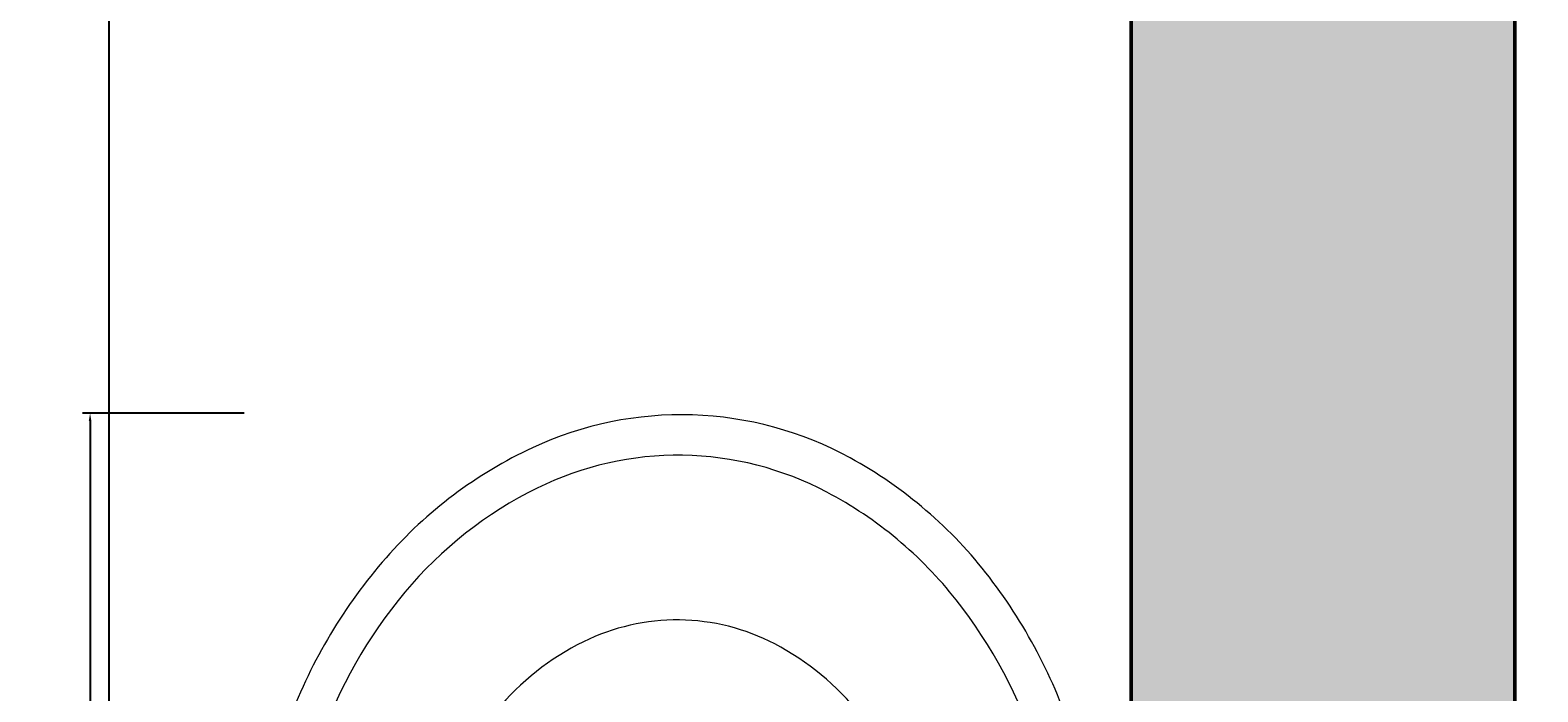
# Model space of a CAD drawing. Units: inches. Extents: x 2307 to 2544, y 2171 to 2540.
# Tile 43 of 52: x 2490 to 2525, y 2466 to 2482. Entities that reach past the tile are written whole.
import ezdxf

# ---------------------------------------------------------------- set-up
doc = ezdxf.new("R2010")
doc.units = ezdxf.units.IN
for name, color, linetype, lineweight in [('A-ANNO-DIMS', 2, 'Continuous', 18), ('A-DOOR', 3, 'Continuous', 25), ('A-FLOR-FIXT', 9, 'Continuous', 18), ('A-WALL', 7, 'Continuous', 50)]:
    doc.layers.add(name, color=color, linetype=linetype, lineweight=lineweight)
doc.layers.add('A-WALL-PATT', color=18, linetype='Continuous', lineweight=13, true_color=0x000000)
doc.styles.get("Standard").update_dxf_attribs({"font": 'arial.ttf'})
doc.dimstyles.get("Standard").update_dxf_attribs({"dimtxt": 0.18, "dimasz": 0.18, "dimexe": 0.18, "dimexo": 0.0625, "dimgap": 0.09, "dimtad": 0, "dimtih": 1, "dimtoh": 1, "dimdec": 4, "dimzin": 0, "dimdsep": 46, "dimtxsty": 'Standard', "dimcen": 0.09, "dimadec": 0, "dimazin": 0, "dimtfac": 1, "dimtdec": 4, "dimtofl": 0, "dimtmove": 0, "dimatfit": 3, "dimfxl": 1, "dimtolj": 1, "dimtzin": 0, "dimarcsym": 0})

# ---------------------------------------------------------------- blocks, each defined once
blk = doc.blocks.new('Sink - Oval top')
for p, q in [((0, 1), (0, -1)), ((-1, 0), (1, 0))]:
    blk.add_line(p, q)
for points in [[(-12.234, 0.394, 0.117634), (-11.465, -3.362, 0.104469), (-8.879, -6.804, 0.090016), (-5.083, -9.072, 0.08192), (-0.323, -10.016, 0.08192), (4.488, -9.381, 0.090016), (8.422, -7.361, 0.104469), (11.224, -4.093, 0.117634), (12.234, -0.394, 0.117634), (11.465, 3.362, 0.104469), (8.879, 6.804, 0.090016), (5.083, 9.072, 0.08192), (0.323, 10.016, 0.08192), (-4.488, 9.381, 0.090016), (-8.422, 7.361, 0.104469), (-11.224, 4.093, 0.117634)], [(-11.286, 0.159, 0.118622), (-10.516, -3.253, 0.104678), (-8.072, -6.359, 0.089562), (-4.538, -8.367, 0.081185), (-0.129, -9.152, 0.081185), (4.3, -8.492, 0.089562), (7.889, -6.584, 0.104678), (10.42, -3.548, 0.118622), (11.286, -0.159, 0.118622), (10.516, 3.253, 0.104678), (8.072, 6.359, 0.089562), (4.538, 8.367, 0.081185), (0.129, 9.152, 0.081185), (-4.3, 8.492, 0.089562), (-7.889, 6.584, 0.104678), (-10.42, 3.548, 0.118622)], [(-7.42, 0.083, 0.118283), (-6.907, -2.167, 0.104607), (-5.295, -4.21, 0.089718), (-2.967, -5.528, 0.081436), (-0.068, -6.037, 0.081436), (2.842, -5.593, 0.089718), (5.199, -4.327, 0.104607), (6.857, -2.321, 0.118283), (7.42, -0.083, 0.118283), (6.907, 2.167, 0.104607), (5.295, 4.21, 0.089718), (2.967, 5.528, 0.081436), (0.068, 6.037, 0.081436), (-2.842, 5.593, 0.089718), (-5.199, 4.327, 0.104607), (-6.857, 2.321, 0.118283)]]:
    blk.add_lwpolyline(points, format="xyb", close=True)
for radius in [1.5, 1]:
    blk.add_circle((0, 0), radius)
blk = doc.blocks.new('*U13')
for p, q in [((0, 0), (0, -6)), ((40, 0), (40, -6))]:
    blk.add_line(p, q)
blk.add_lwpolyline([(0, 0), (0, 40), (1.75, 40), (1.75, 0)], close=True)
blk.add_arc((0, 0), 40, 0, 90)
blk = doc.blocks.new('*D22')
at = {"layer": 'A-ANNO-DIMS', "color": 0, "lineweight": -2, "transparency": 16777216}
for p, q in [((2494.871, 2472.93), (2491.071, 2472.93)), ((2491.251, 2472.75), (2491.251, 2460.838)), ((2491.251, 2448.56), (2491.251, 2460.472)), ((2494.871, 2448.38), (2491.071, 2448.38))]:
    blk.add_line(p, q, dxfattribs=at)
at = {"layer": 'A-ANNO-DIMS', "color": 0, "transparency": 16777216}
for points in [[(2491.221, 2472.75), (2491.281, 2472.75), (2491.251, 2472.93)], [(2491.221, 2448.56), (2491.281, 2448.56), (2491.251, 2448.38)]]:
    blk.add_solid(points, dxfattribs=at)
at = {"layer": 'Defpoints', "color": 0, "transparency": 16777216}
for p in [(2494.934, 2472.93), (2491.251, 2448.38), (2494.934, 2448.38)]:
    blk.add_point(p, dxfattribs=at)
at = {"layer": 'A-ANNO-DIMS', "color": 0, "transparency": 16777216, "insert": (2491.251, 2460.655), "char_height": 0.18, "attachment_point": 5}
blk.add_mtext('\\A1;BASIN 25', dxfattribs=at)
blk = doc.blocks.new('*D37')
at = {"layer": 'A-ANNO-DIMS', "color": 0, "lineweight": -2, "transparency": 16777216}
for p, q in [((2524.758, 2520.51), (2544.026, 2520.51)), ((2543.846, 2520.33), (2543.846, 2355.692)), ((2543.846, 2190.69), (2543.846, 2355.328)), ((2524.758, 2190.51), (2544.026, 2190.51))]:
    blk.add_line(p, q, dxfattribs=at)
at = {"layer": 'A-ANNO-DIMS', "color": 0, "transparency": 16777216}
for points in [[(2543.816, 2520.33), (2543.876, 2520.33), (2543.846, 2520.51)], [(2543.816, 2190.69), (2543.876, 2190.69), (2543.846, 2190.51)]]:
    blk.add_solid(points, dxfattribs=at)
at = {"layer": 'Defpoints', "color": 0, "transparency": 16777216}
for p in [(2524.696, 2520.51), (2543.846, 2520.51), (2524.696, 2190.51)]:
    blk.add_point(p, dxfattribs=at)
at = {"layer": 'A-ANNO-DIMS', "color": 0, "transparency": 16777216, "insert": (2543.846, 2355.51), "char_height": 0.18, "attachment_point": 5}
blk.add_mtext('\\A1;330', dxfattribs=at)
blk = doc.blocks.new('*D61')
at = {"layer": 'A-ANNO-DIMS', "color": 0, "lineweight": -2, "transparency": 16777216}
for p, q in [((2491.696, 2435.572), (2491.696, 2540.345)), ((2491.876, 2540.165), (2503.476, 2540.165)), ((2515.516, 2540.165), (2503.916, 2540.165)), ((2515.696, 2435.572), (2515.696, 2540.345))]:
    blk.add_line(p, q, dxfattribs=at)
at = {"layer": 'A-ANNO-DIMS', "color": 0, "transparency": 16777216}
for points in [[(2491.876, 2540.195), (2491.876, 2540.135), (2491.696, 2540.165)], [(2515.516, 2540.195), (2515.516, 2540.135), (2515.696, 2540.165)]]:
    blk.add_solid(points, dxfattribs=at)
at = {"layer": 'Defpoints', "color": 0, "transparency": 16777216}
for p in [(2515.696, 2540.165), (2491.696, 2435.51), (2515.696, 2435.51)]:
    blk.add_point(p, dxfattribs=at)
at = {"layer": 'A-ANNO-DIMS', "color": 0, "transparency": 16777216, "insert": (2503.696, 2540.165), "char_height": 0.18, "attachment_point": 5}
blk.add_mtext('\\A1;24', dxfattribs=at)

msp = doc.modelspace()

# ---------------------------------------------------------------- hatches: boundary and pattern name
at = {"layer": 'A-WALL-PATT'}
h = msp.add_hatch(color=256, dxfattribs=at)
h.dxf.hatch_style = 1
h.paths.add_polyline_path([(2433.6935, 2199.5096), (2415.6423, 2199.5096), (2415.6423, 2190.5096), (2433.7832, 2190.5096)], flags=17)
h.paths.add_polyline_path([(2367.6423, 2199.5096), (2335.6958, 2199.5096), (2335.6958, 2307.3983), (2326.6958, 2307.3983), (2326.6958, 2190.5096), (2367.6423, 2190.5096)])
h.paths.add_polyline_path([(2524.6958, 2520.5096), (2496.7832, 2520.5096), (2496.7832, 2515.5149), (2472.7832, 2515.5149), (2472.7832, 2520.5096), (2415.4028, 2520.5096), (2415.4028, 2511.5096), (2451.6958, 2511.5096), (2451.6958, 2439.5096), (2451.6958, 2391.5096), (2445.6958, 2391.5096), (2445.6958, 2387.5096), (2455.6958, 2387.5096), (2455.6958, 2435.5096), (2461.6958, 2435.5096), (2461.6958, 2439.5096), (2455.6958, 2439.5096), (2455.6958, 2511.5096), (2515.6958, 2511.5096), (2515.6958, 2439.5096), (2491.6958, 2439.5096), (2491.6958, 2435.5096), (2515.6958, 2435.5096), (2515.6958, 2319.5096), (2451.6958, 2319.5096), (2451.6958, 2281.5096), (2481.6958, 2281.5096), (2481.6958, 2225.5096), (2485.6958, 2225.5096), (2485.6958, 2285.5096), (2455.6958, 2285.5096), (2455.6958, 2315.5096), (2515.6958, 2315.5096), (2515.6958, 2199.5096), (2469.6952, 2199.5096), (2469.785, 2190.5096), (2524.6958, 2190.5096)])

# ---------------------------------------------------------------- linework, layer by layer
at = {"layer": 'A-WALL'}
msp.add_line((2515.6958, 2511.5096), (2515.6958, 2439.5096), dxfattribs=at)
msp.add_lwpolyline([(2433.7832, 2190.5096), (2326.6958, 2190.5096), (2326.6958, 2520.5096), (2524.6958, 2520.5096), (2524.6958, 2190.5096), (2469.785, 2190.5096)], dxfattribs=at)

# ---------------------------------------------------------------- block references
at = {"layer": 'A-DOOR', "xscale": 0.75, "yscale": 0.75, "zscale": 0.75}
msp.add_blockref('*U13', (2461.6958, 2440.0096), dxfattribs=at)
at = {"layer": 'A-FLOR-FIXT', "rotation": 270}
msp.add_blockref('Sink - Oval top', (2505.002, 2460.655), dxfattribs=at)

# ---------------------------------------------------------------- dimensions: what is measured, and where the dimension line sits
at = {"layer": 'A-ANNO-DIMS'}
dim = msp.add_linear_dim(base=(2515.6958, 2540.1649), p1=(2491.6958, 2435.5096), p2=(2515.6958, 2435.5096), dimstyle='Standard', override={"dimdec": 0, "dimlfac": 1, "dimrnd": 0, "dimzin": 0, "dimdsep": 46, "dimlunit": 2}, dxfattribs=at)
dim.commit()
dim.dimension.update_dxf_attribs({"geometry": '*D61', "text_midpoint": (2503.6958, 2540.1649)})
dim = msp.add_linear_dim(base=(2543.8458, 2520.5096), p1=(2524.6958, 2190.5096), p2=(2524.6958, 2520.5096), angle=90, dimstyle='Standard', override={"dimdec": 0, "dimlfac": 1, "dimrnd": 0, "dimzin": 0, "dimdsep": 46, "dimlunit": 2}, dxfattribs=at)
dim.commit()
dim.dimension.update_dxf_attribs({"geometry": '*D37', "text_midpoint": (2543.8458, 2355.5096)})
dim = msp.add_linear_dim(base=(2491.2511, 2448.3795), p1=(2494.9337, 2472.9304), p2=(2494.9337, 2448.3795), angle=270, text='BASIN <>', dimstyle='Standard', override={"dimdec": 0, "dimlfac": 1, "dimrnd": 0, "dimzin": 0, "dimdsep": 46, "dimlunit": 2}, dxfattribs=at)
dim.commit()
dim.dimension.update_dxf_attribs({"geometry": '*D22', "text_midpoint": (2491.2511, 2460.655)})

doc.saveas('drawing.dxf')
